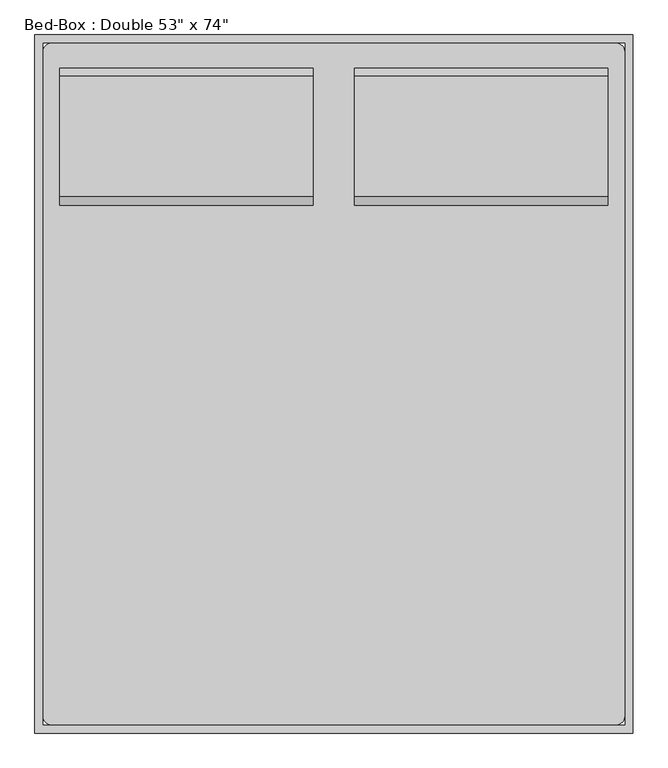
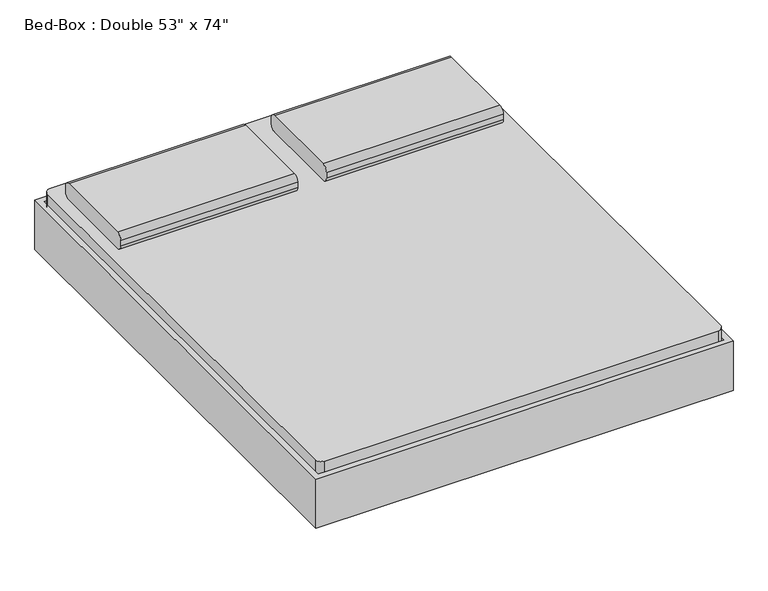
"""IFC4 building model written with IfcOpenShell, lengths in millimetres: furniture geometry."""

from ifc_helpers import new_model, si_unit, point, frame, frame_2d, origin, place, context, project, spatial, polyline, circle_curve, trimmed, segment, composite_curve, outline, extrude, source, transform, mapped, element, save
from ifc_brep_helpers import plane_surface, cylinder_surface, revolved_surface, advanced_brep


def furniture_2b620373(model_context):
    return source(origin(), model_context, "Body", "SolidModel", [
        extrude(outline(composite_curve([segment(polyline([(705.3704918, 406.4), (337.0704918, 406.4)]), True, "CONTINUOUS"), segment(trimmed(circle_curve(frame_2d((337.0704918, 431.8)), 25.4), [point((337.0704918, 406.4))], [point((311.6704918, 431.8))], False, "CARTESIAN"), True, "CONTINUOUS"), segment(polyline([(311.6704918, 431.8), (311.6704918, 457.2)]), True, "CONTINUOUS"), segment(trimmed(circle_curve(frame_2d((337.0704918, 457.2)), 25.4), [point((311.6704918, 457.2))], [point((337.0704918, 482.6))], False, "CARTESIAN"), True, "CONTINUOUS"), segment(polyline([(337.0704918, 482.6), (705.3704918, 482.6)]), True, "CONTINUOUS"), segment(trimmed(circle_curve(frame_2d((705.3704918, 457.2)), 25.4), [point((705.3704918, 482.6))], [point((730.7704918, 457.2))], False, "CARTESIAN"), True, "CONTINUOUS"), segment(polyline([(730.7704918, 457.2), (730.7704918, 431.8)]), True, "CONTINUOUS"), segment(trimmed(circle_curve(frame_2d((705.3704918, 431.8)), 25.4), [point((730.7704918, 431.8))], [point((705.3704918, 406.4))], False, "CARTESIAN"), True, "CONTINUOUS")], self_intersect=False)), frame((402.652459, 0.0, 0.0), z_axis=(1.0, 0.0, 0.0), x_axis=(0.0, 1.0, 0.0)), (0.0, 0.0, 1.0), 774.7),
        extrude(outline(composite_curve([segment(polyline([(705.3704918, 406.4), (337.0704918, 406.4)]), True, "CONTINUOUS"), segment(trimmed(circle_curve(frame_2d((337.0704918, 431.8)), 25.4), [point((337.0704918, 406.4))], [point((311.6704918, 431.8))], False, "CARTESIAN"), True, "CONTINUOUS"), segment(polyline([(311.6704918, 431.8), (311.6704918, 457.2)]), True, "CONTINUOUS"), segment(trimmed(circle_curve(frame_2d((337.0704918, 457.2)), 25.4), [point((311.6704918, 457.2))], [point((337.0704918, 482.6))], False, "CARTESIAN"), True, "CONTINUOUS"), segment(polyline([(337.0704918, 482.6), (705.3704918, 482.6)]), True, "CONTINUOUS"), segment(trimmed(circle_curve(frame_2d((705.3704918, 457.2)), 25.4), [point((705.3704918, 482.6))], [point((730.7704918, 457.2))], False, "CARTESIAN"), True, "CONTINUOUS"), segment(polyline([(730.7704918, 457.2), (730.7704918, 431.8)]), True, "CONTINUOUS"), segment(trimmed(circle_curve(frame_2d((705.3704918, 431.8)), 25.4), [point((730.7704918, 431.8))], [point((705.3704918, 406.4))], False, "CARTESIAN"), True, "CONTINUOUS")], self_intersect=False)), frame((-499.047541, 0.0, 0.0), z_axis=(1.0, 0.0, 0.0), x_axis=(0.0, 1.0, 0.0)), (0.0, 0.0, 1.0), 774.7),
        advanced_brep(
        [(-549.5231784, 578.3704918, 177.8), (-549.5231784, 502.1704918, 177.8), (-549.5231784, 502.1704918, 196.85), (-549.5231784, 578.3704918, 196.85), (-498.7231784, 578.3704918, 177.8), (-498.7231784, 502.1704918, 177.8), (-486.5869899, 502.1704918, 196.85), (-486.5869899, 578.3704918, 196.85), (-422.6523099, 578.3704918, 14.6654962), (-422.6523099, 502.1704918, 14.6654962), (-405.3871466, 502.1704918, 22.716374), (-405.3871466, 578.3704918, 22.716374), (-399.6320921, 502.1704918, 0.0), (-399.6320921, 578.3704918, 0.0), (-399.6320921, 502.1704918, 19.05), (-399.6320921, 578.3704918, 19.05), (-321.0195862, 578.3704918, 0.0), (-321.0195862, 502.1704918, 0.0), (-321.0195862, 502.1704918, 19.05), (-321.0195862, 578.3704918, 19.05), (-308.3195862, 502.1704918, 3.4029547), (-308.3195862, 578.3704918, 3.4029547), (-317.8445862, 502.1704918, 19.9007387), (-317.8445862, 578.3704918, 19.9007387), (-248.222541, 578.3704918, 38.1), (-248.222541, 502.1704918, 38.1), (-253.3269731, 502.1704918, 57.15), (-253.3269731, 578.3704918, 57.15), (926.8518216, 578.3704918, 38.1), (926.8518216, 502.1704918, 38.1), (931.9562537, 502.1704918, 57.15), (931.9562537, 578.3704918, 57.15), (986.9488669, 578.3704918, 3.4029547), (986.9488669, 502.1704918, 3.4029547), (996.4738669, 502.1704918, 19.9007387), (996.4738669, 578.3704918, 19.9007387), (999.6488669, 502.1704918, 0.0), (999.6488669, 578.3704918, 0.0), (999.6488669, 502.1704918, 19.05), (999.6488669, 578.3704918, 19.05), (1078.2613728, 578.3704918, 0.0), (1078.2613728, 502.1704918, 0.0), (1078.2613728, 502.1704918, 19.05), (1078.2613728, 578.3704918, 19.05), (1101.2815906, 502.1704918, 14.6654962), (1101.2815906, 578.3704918, 14.6654962), (1084.0164272, 502.1704918, 22.716374), (1084.0164272, 578.3704918, 22.716374), (1177.352459, 578.3704918, 177.8), (1177.352459, 502.1704918, 177.8), (1165.2162705, 502.1704918, 196.85), (1165.2162705, 578.3704918, 196.85), (1228.152459, 578.3704918, 177.8), (1228.152459, 578.3704918, 196.85), (1228.152459, 502.1704918, 196.85), (1228.152459, 502.1704918, 177.8)],
        [
            (0, 1),
            (1, 2),
            (2, 3),
            (3, 0),
            (0, 4),
            (4, 5),
            (5, 1),
            (5, 6),
            (6, 2),
            (6, 7),
            (7, 3),
            (7, 4),
            (4, 8),
            (8, 9),
            (9, 5),
            (9, 10),
            (10, 6),
            (10, 11),
            (11, 7),
            (11, 8),
            (12, 9, circle_curve(frame((-399.6320921, 502.1704918, 25.4), z_axis=(0.0, 1.0, 0.0), x_axis=(-0.9063077870366486, 0.0, -0.42261826174070233)), 25.4)),
            (8, 13, circle_curve(frame((-399.6320921, 578.3704918, 25.4), z_axis=(0.0, -1.0, 0.0), x_axis=(-0.9063077870366486, 0.0, -0.42261826174070233)), 25.4)),
            (13, 12),
            (14, 10, circle_curve(frame((-399.6320921, 502.1704918, 25.4), z_axis=(0.0, 1.0, 0.0), x_axis=(-0.9063077870366486, 0.0, -0.42261826174070233)), 6.35)),
            (12, 14),
            (15, 11, circle_curve(frame((-399.6320921, 578.3704918, 25.4), z_axis=(0.0, 1.0, 0.0), x_axis=(-0.9063077870366486, 0.0, -0.42261826174070233)), 6.35)),
            (14, 15),
            (15, 13),
            (13, 16),
            (16, 17),
            (17, 12),
            (17, 18),
            (18, 14),
            (18, 19),
            (19, 15),
            (19, 16),
            (20, 17, circle_curve(frame((-321.0195862, 502.1704918, 25.4), z_axis=(0.0, 1.0, 0.0), x_axis=(0.0, 0.0, -1.0)), 25.4)),
            (16, 21, circle_curve(frame((-321.0195862, 578.3704918, 25.4), z_axis=(0.0, -1.0, 0.0), x_axis=(0.0, 0.0, -1.0)), 25.4)),
            (21, 20),
            (22, 18, circle_curve(frame((-321.0195862, 502.1704918, 25.4), z_axis=(0.0, 1.0, 0.0), x_axis=(0.0, 0.0, -1.0)), 6.35)),
            (20, 22),
            (23, 19, circle_curve(frame((-321.0195862, 578.3704918, 25.4), z_axis=(0.0, 1.0, 0.0), x_axis=(0.0, 0.0, -1.0)), 6.35)),
            (22, 23),
            (23, 21),
            (21, 24),
            (24, 25),
            (25, 20),
            (25, 26),
            (26, 22),
            (26, 27),
            (27, 23),
            (27, 24),
            (24, 28),
            (28, 29),
            (29, 25),
            (29, 30),
            (30, 26),
            (30, 31),
            (31, 27),
            (31, 28),
            (28, 32),
            (32, 33),
            (33, 29),
            (33, 34),
            (34, 30),
            (34, 35),
            (35, 31),
            (35, 32),
            (36, 33, circle_curve(frame((999.6488669, 502.1704918, 25.4), z_axis=(0.0, 1.0, 0.0), x_axis=(-0.5000000000000463, 0.0, -0.8660254037844118)), 25.4)),
            (32, 37, circle_curve(frame((999.6488669, 578.3704918, 25.4), z_axis=(0.0, -1.0, 0.0), x_axis=(-0.5000000000000463, 0.0, -0.8660254037844118)), 25.4)),
            (37, 36),
            (38, 34, circle_curve(frame((999.6488669, 502.1704918, 25.4), z_axis=(0.0, 1.0, 0.0), x_axis=(-0.5000000000000463, 0.0, -0.8660254037844118)), 6.35)),
            (36, 38),
            (39, 35, circle_curve(frame((999.6488669, 578.3704918, 25.4), z_axis=(0.0, 1.0, 0.0), x_axis=(-0.5000000000000463, 0.0, -0.8660254037844118)), 6.35)),
            (38, 39),
            (39, 37),
            (37, 40),
            (40, 41),
            (41, 36),
            (41, 42),
            (42, 38),
            (42, 43),
            (43, 39),
            (43, 40),
            (44, 41, circle_curve(frame((1078.2613728, 502.1704918, 25.4), z_axis=(0.0, 1.0, 0.0), x_axis=(0.0, 0.0, -1.0)), 25.4)),
            (40, 45, circle_curve(frame((1078.2613728, 578.3704918, 25.4), z_axis=(0.0, -1.0, 0.0), x_axis=(0.0, 0.0, -1.0)), 25.4)),
            (45, 44),
            (46, 42, circle_curve(frame((1078.2613728, 502.1704918, 25.4), z_axis=(0.0, 1.0, 0.0), x_axis=(0.0, 0.0, -1.0)), 6.35)),
            (44, 46),
            (47, 43, circle_curve(frame((1078.2613728, 578.3704918, 25.4), z_axis=(0.0, 1.0, 0.0), x_axis=(0.0, 0.0, -1.0)), 6.35)),
            (46, 47),
            (47, 45),
            (45, 48),
            (48, 49),
            (49, 44),
            (49, 50),
            (50, 46),
            (50, 51),
            (51, 47),
            (51, 48),
            (52, 53),
            (53, 54),
            (54, 55),
            (55, 52),
            (48, 52),
            (55, 49),
            (54, 50),
            (53, 51),
        ],
        [
            plane_surface(frame((-549.5231784, 832.3704918, -152.9490627), z_axis=(-1.0, 0.0, 0.0), x_axis=(0.0, 1.0, 0.0))),
            plane_surface(frame((-549.5231784, 578.3704918, 177.8), z_axis=(0.0, 0.0, -1.0), x_axis=(1.0, 0.0, 0.0))),
            plane_surface(frame((-549.5231784, 502.1704918, 177.8), z_axis=(0.0, -1.0, 0.0), x_axis=(1.0, 0.0, 0.0))),
            plane_surface(frame((-549.5231784, 502.1704918, 196.85), z_axis=(0.0, 0.0, 1.0), x_axis=(1.0, 0.0, 0.0))),
            plane_surface(frame((-549.5231784, 578.3704918, 196.85), z_axis=(0.0, 1.0, 0.0), x_axis=(1.0, 0.0, 0.0))),
            plane_surface(frame((-498.7231784, 578.3704918, 177.8), z_axis=(-0.9063077870366487, 0.0, -0.4226182617407023), x_axis=(0.4226182617407023, 0.0, -0.9063077870366487))),
            plane_surface(frame((-498.7231784, 502.1704918, 177.8), z_axis=(0.0, -1.0000000000000002, 0.0), x_axis=(0.4226182617407023, 0.0, -0.9063077870366487))),
            plane_surface(frame((-486.5869899, 502.1704918, 196.85), z_axis=(0.9063077870366488, 0.0, 0.42261826174070205), x_axis=(0.42261826174070205, 0.0, -0.9063077870366488))),
            plane_surface(frame((-486.5869899, 578.3704918, 196.85), z_axis=(0.0, 1.0000000000000002, 0.0), x_axis=(0.4226182617407021, 0.0, -0.9063077870366487))),
            cylinder_surface(frame((-399.6320921, 832.3704918, 25.4), z_axis=(0.0, -1.0, 0.0), x_axis=(-0.9063077870366486, 0.0, -0.42261826174070233)), 25.4),
            plane_surface(frame((-399.6320921, 502.1704918, 25.4), z_axis=(0.0, -1.0, 0.0), x_axis=(-0.9063077870366486, 0.0, -0.42261826174070233))),
            revolved_surface(polyline([(-405.38714654768273, 502.1704918, 22.71637403794654), (-405.38714654768273, 578.3704918, 22.71637403794654)]), (-399.6320921, 832.3704918, 25.4), (0.0, -1.0, 0.0)),
            plane_surface(frame((-399.6320921, 578.3704918, 25.4), z_axis=(0.0, 1.0, 0.0), x_axis=(-0.9063077870366486, 0.0, -0.42261826174070233))),
            plane_surface(frame((-399.6320921, 578.3704918, 0.0), z_axis=(0.0, 0.0, -1.0), x_axis=(1.0, 0.0, 0.0))),
            plane_surface(frame((-399.6320921, 502.1704918, 0.0), z_axis=(0.0, -1.0, 0.0), x_axis=(1.0, 0.0, 0.0))),
            plane_surface(frame((-399.6320921, 502.1704918, 19.05), z_axis=(0.0, 0.0, 1.0), x_axis=(1.0, 0.0, 0.0))),
            plane_surface(frame((-399.6320921, 578.3704918, 19.05), z_axis=(0.0, 1.0, 0.0), x_axis=(1.0, 0.0, 0.0))),
            cylinder_surface(frame((-321.0195862, 832.3704918, 25.4), z_axis=(0.0, -1.0, 0.0), x_axis=(0.0, 0.0, -1.0)), 25.4),
            plane_surface(frame((-321.0195862, 502.1704918, 25.4), z_axis=(0.0, -1.0, 0.0), x_axis=(0.0, 0.0, -1.0))),
            revolved_surface(polyline([(-321.0195862, 502.1704918, 19.049999999999997), (-321.0195862, 578.3704918, 19.049999999999997)]), (-321.0195862, 832.3704918, 25.4), (0.0, -1.0, 0.0)),
            plane_surface(frame((-321.0195862, 578.3704918, 25.4), z_axis=(0.0, 1.0, 0.0), x_axis=(0.0, 0.0, -1.0))),
            plane_surface(frame((-308.3195862, 578.3704918, 3.4029547), z_axis=(0.49999999999987804, 0.0, -0.8660254037845091), x_axis=(0.8660254037845091, 0.0, 0.49999999999987804))),
            plane_surface(frame((-308.3195862, 502.1704918, 3.4029547), z_axis=(0.0, -1.0000000000000002, 0.0), x_axis=(0.8660254037845095, 0.0, 0.4999999999998774))),
            plane_surface(frame((-317.8445862, 502.1704918, 19.9007387), z_axis=(-0.49999999999987743, 0.0, 0.8660254037845095), x_axis=(0.8660254037845095, 0.0, 0.49999999999987743))),
            plane_surface(frame((-317.8445862, 578.3704918, 19.9007387), z_axis=(0.0, 1.0, 0.0), x_axis=(0.8660254037845087, 0.0, 0.49999999999987876))),
            plane_surface(frame((-248.222541, 578.3704918, 38.1), z_axis=(0.0, 0.0, -1.0), x_axis=(1.0, 0.0, 0.0))),
            plane_surface(frame((-248.222541, 502.1704918, 38.1), z_axis=(0.0, -1.0, 0.0), x_axis=(1.0, 0.0, 0.0))),
            plane_surface(frame((-253.3269731, 502.1704918, 57.15), z_axis=(0.0, 0.0, 1.0), x_axis=(1.0, 0.0, 0.0))),
            plane_surface(frame((-253.3269731, 578.3704918, 57.15), z_axis=(0.0, 1.0, 0.0), x_axis=(1.0, 0.0, 0.0))),
            plane_surface(frame((926.8518216, 578.3704918, 38.1), z_axis=(-0.5000000000000462, 0.0, -0.866025403784412), x_axis=(0.866025403784412, 0.0, -0.5000000000000462))),
            plane_surface(frame((926.8518216, 502.1704918, 38.1), z_axis=(0.0, -1.0, 0.0), x_axis=(0.8660254037844121, 0.0, -0.5000000000000461))),
            plane_surface(frame((931.9562537, 502.1704918, 57.15), z_axis=(0.5000000000000455, 0.0, 0.8660254037844124), x_axis=(0.8660254037844124, 0.0, -0.5000000000000455))),
            plane_surface(frame((931.9562537, 578.3704918, 57.15), z_axis=(0.0, 1.0, 0.0), x_axis=(0.866025403784413, 0.0, -0.5000000000000446))),
            cylinder_surface(frame((999.6488669, 832.3704918, 25.4), z_axis=(0.0, -1.0, 0.0), x_axis=(-0.5000000000000463, 0.0, -0.8660254037844118)), 25.4),
            plane_surface(frame((999.6488669, 502.1704918, 25.4), z_axis=(0.0, -1.0000000000000002, 0.0), x_axis=(-0.5000000000000464, 0.0, -0.866025403784412))),
            revolved_surface(polyline([(996.4738668999997, 502.1704918, 19.90073868596898), (996.4738668999997, 578.3704918, 19.90073868596898)]), (999.6488669, 832.3704918, 25.4), (0.0, -1.0, 0.0)),
            plane_surface(frame((999.6488669, 578.3704918, 25.4), z_axis=(0.0, 1.0000000000000002, 0.0), x_axis=(-0.5000000000000464, 0.0, -0.866025403784412))),
            plane_surface(frame((999.6488669, 578.3704918, 0.0), z_axis=(0.0, 0.0, -1.0), x_axis=(1.0, 0.0, 0.0))),
            plane_surface(frame((999.6488669, 502.1704918, 0.0), z_axis=(0.0, -1.0, 0.0), x_axis=(1.0, 0.0, 0.0))),
            plane_surface(frame((999.6488669, 502.1704918, 19.05), z_axis=(0.0, 0.0, 1.0), x_axis=(1.0, 0.0, 0.0))),
            plane_surface(frame((999.6488669, 578.3704918, 19.05), z_axis=(0.0, 1.0, 0.0), x_axis=(1.0, 0.0, 0.0))),
            cylinder_surface(frame((1078.2613728, 832.3704918, 25.4), z_axis=(0.0, -1.0, 0.0), x_axis=(0.0, 0.0, -1.0)), 25.4),
            plane_surface(frame((1078.2613728, 502.1704918, 25.4), z_axis=(0.0, -1.0, 0.0), x_axis=(0.0, 0.0, -1.0))),
            revolved_surface(polyline([(1078.2613728, 502.1704918, 19.049999999999997), (1078.2613728, 578.3704918, 19.049999999999997)]), (1078.2613728, 832.3704918, 25.4), (0.0, -1.0, 0.0)),
            plane_surface(frame((1078.2613728, 578.3704918, 25.4), z_axis=(0.0, 1.0, 0.0), x_axis=(0.0, 0.0, -1.0))),
            plane_surface(frame((1101.2815906, 578.3704918, 14.6654962), z_axis=(0.90630778703668, 0.0, -0.422618261740635), x_axis=(0.422618261740635, 0.0, 0.90630778703668))),
            plane_surface(frame((1101.2815906, 502.1704918, 14.6654962), z_axis=(0.0, -1.0000000000000002, 0.0), x_axis=(0.4226182617406349, 0.0, 0.9063077870366801))),
            plane_surface(frame((1084.0164272, 502.1704918, 22.716374), z_axis=(-0.9063077870366799, 0.0, 0.4226182617406352), x_axis=(0.4226182617406352, 0.0, 0.9063077870366799))),
            plane_surface(frame((1084.0164272, 578.3704918, 22.716374), z_axis=(0.0, 1.0, 0.0), x_axis=(0.42261826174063544, 0.0, 0.9063077870366798))),
            plane_surface(frame((1228.152459, 832.3704918, -152.9490627), z_axis=(1.0, 0.0, 0.0), x_axis=(0.0, 1.0, 0.0))),
            plane_surface(frame((1177.352459, 578.3704918, 177.8), z_axis=(0.0, 0.0, -1.0), x_axis=(1.0, 0.0, 0.0))),
            plane_surface(frame((1177.352459, 502.1704918, 177.8), z_axis=(0.0, -1.0, 0.0), x_axis=(1.0, 0.0, 0.0))),
            plane_surface(frame((1165.2162705, 502.1704918, 196.85), z_axis=(0.0, 0.0, 1.0), x_axis=(1.0, 0.0, 0.0))),
            plane_surface(frame((1165.2162705, 578.3704918, 196.85), z_axis=(0.0, 1.0, 0.0), x_axis=(1.0, 0.0, 0.0))),
        ],
        [
            (0, [[1, 2, 3, 4]]),
            (1, [[-1, 5, 6, 7]]),
            (2, [[-2, -7, 8, 9]]),
            (3, [[-3, -9, 10, 11]]),
            (4, [[-4, -11, 12, -5]]),
            (5, [[-6, 13, 14, 15]]),
            (6, [[-8, -15, 16, 17]]),
            (7, [[-10, -17, 18, 19]]),
            (8, [[-12, -19, 20, -13]]),
            (9, [[21, -14, 22, 23]]),
            (10, [[24, -16, -21, 25]]),
            (11, [[26, -18, -24, 27]]),
            (12, [[-22, -20, -26, 28]]),
            (13, [[-23, 29, 30, 31]]),
            (14, [[-25, -31, 32, 33]]),
            (15, [[-27, -33, 34, 35]]),
            (16, [[-28, -35, 36, -29]]),
            (17, [[37, -30, 38, 39]]),
            (18, [[40, -32, -37, 41]]),
            (19, [[42, -34, -40, 43]]),
            (20, [[-38, -36, -42, 44]]),
            (21, [[-39, 45, 46, 47]]),
            (22, [[-41, -47, 48, 49]]),
            (23, [[-43, -49, 50, 51]]),
            (24, [[-44, -51, 52, -45]]),
            (25, [[-46, 53, 54, 55]]),
            (26, [[-48, -55, 56, 57]]),
            (27, [[-50, -57, 58, 59]]),
            (28, [[-52, -59, 60, -53]]),
            (29, [[-54, 61, 62, 63]]),
            (30, [[-56, -63, 64, 65]]),
            (31, [[-58, -65, 66, 67]]),
            (32, [[-60, -67, 68, -61]]),
            (33, [[69, -62, 70, 71]]),
            (34, [[72, -64, -69, 73]]),
            (35, [[74, -66, -72, 75]]),
            (36, [[-70, -68, -74, 76]]),
            (37, [[-71, 77, 78, 79]]),
            (38, [[-73, -79, 80, 81]]),
            (39, [[-75, -81, 82, 83]]),
            (40, [[-76, -83, 84, -77]]),
            (41, [[85, -78, 86, 87]]),
            (42, [[88, -80, -85, 89]]),
            (43, [[90, -82, -88, 91]]),
            (44, [[-86, -84, -90, 92]]),
            (45, [[-87, 93, 94, 95]]),
            (46, [[-89, -95, 96, 97]]),
            (47, [[-91, -97, 98, 99]]),
            (48, [[-92, -99, 100, -93]]),
            (49, [[101, 102, 103, 104]]),
            (50, [[-94, 105, -104, 106]]),
            (51, [[-96, -106, -103, 107]]),
            (52, [[-98, -107, -102, 108]]),
            (53, [[-100, -108, -101, -105]]),
        ],
    ),
        extrude(outline(composite_curve([segment(polyline([(-524.447541, 806.9704918), (1202.752459, 806.9704918)]), True, "CONTINUOUS"), segment(trimmed(circle_curve(frame_2d((1202.752459, 781.5704918)), 25.4), [point((1202.752459, 806.9704918))], [point((1228.152459, 781.5704918))], False, "CARTESIAN"), True, "CONTINUOUS"), segment(polyline([(1228.152459, 781.5704918), (1228.152459, -1250.4295082)]), True, "CONTINUOUS"), segment(trimmed(circle_curve(frame_2d((1202.752459, -1250.4295082)), 25.4), [point((1228.152459, -1250.4295082))], [point((1202.752459, -1275.8295082))], False, "CARTESIAN"), True, "CONTINUOUS"), segment(polyline([(1202.752459, -1275.8295082), (-524.447541, -1275.8295082)]), True, "CONTINUOUS"), segment(trimmed(circle_curve(frame_2d((-524.447541, -1250.4295082)), 25.4), [point((-524.447541, -1275.8295082))], [point((-549.847541, -1250.4295082))], False, "CARTESIAN"), True, "CONTINUOUS"), segment(polyline([(-549.847541, -1250.4295082), (-549.847541, 781.5704918)]), True, "CONTINUOUS"), segment(trimmed(circle_curve(frame_2d((-524.447541, 781.5704918)), 25.4), [point((-549.847541, 781.5704918))], [point((-524.447541, 806.9704918))], False, "CARTESIAN"), True, "CONTINUOUS")], self_intersect=False)), frame((0.0, 0.0, 203.2), z_axis=(0.0, 0.0, 1.0), x_axis=(1.0, 0.0, 0.0)), (0.0, 0.0, 1.0), 203.2),
        advanced_brep(
        [(-549.847541, -996.4295082, 196.85), (-549.847541, -996.4295082, 177.8), (-549.847541, -1072.6295082, 177.8), (-549.847541, -1072.6295082, 196.85), (-486.9113525, -996.4295082, 196.85), (-499.047541, -996.4295082, 177.8), (-499.047541, -1072.6295082, 177.8), (-486.9113525, -1072.6295082, 196.85), (-405.7115092, -996.4295082, 22.716374), (-422.9766725, -996.4295082, 14.6654962), (-422.9766725, -1072.6295082, 14.6654962), (-405.7115092, -1072.6295082, 22.716374), (-399.9564547, -996.4295082, 0.0), (-399.9564547, -996.4295082, 19.05), (-399.9564547, -1072.6295082, 0.0), (-399.9564547, -1072.6295082, 19.05), (-321.3439489, -996.4295082, 19.05), (-321.3439489, -996.4295082, 0.0), (-321.3439489, -1072.6295082, 0.0), (-321.3439489, -1072.6295082, 19.05), (-308.6439489, -996.4295082, 3.4029547), (-318.1689489, -996.4295082, 19.9007387), (-308.6439489, -1072.6295082, 3.4029547), (-318.1689489, -1072.6295082, 19.9007387), (-253.6513357, -996.4295082, 57.15), (-248.5469036, -996.4295082, 38.1), (-248.5469036, -1072.6295082, 38.1), (-253.6513357, -1072.6295082, 57.15), (931.9562537, -996.4295082, 57.15), (926.8518216, -996.4295082, 38.1), (926.8518216, -1072.6295082, 38.1), (931.9562537, -1072.6295082, 57.15), (996.4738669, -996.4295082, 19.9007387), (986.9488669, -996.4295082, 3.4029547), (986.9488669, -1072.6295082, 3.4029547), (996.4738669, -1072.6295082, 19.9007387), (999.6488669, -996.4295082, 0.0), (999.6488669, -996.4295082, 19.05), (999.6488669, -1072.6295082, 0.0), (999.6488669, -1072.6295082, 19.05), (1078.2613728, -996.4295082, 19.05), (1078.2613728, -996.4295082, 0.0), (1078.2613728, -1072.6295082, 0.0), (1078.2613728, -1072.6295082, 19.05), (1101.2815906, -996.4295082, 14.6654962), (1084.0164272, -996.4295082, 22.716374), (1101.2815906, -1072.6295082, 14.6654962), (1084.0164272, -1072.6295082, 22.716374), (1165.2162705, -996.4295082, 196.85), (1177.352459, -996.4295082, 177.8), (1177.352459, -1072.6295082, 177.8), (1165.2162705, -1072.6295082, 196.85), (1228.152459, -996.4295082, 196.85), (1228.152459, -1072.6295082, 196.85), (1228.152459, -1072.6295082, 177.8), (1228.152459, -996.4295082, 177.8)],
        [
            (0, 1),
            (1, 2),
            (2, 3),
            (3, 0),
            (0, 4),
            (4, 5),
            (5, 1),
            (5, 6),
            (6, 2),
            (6, 7),
            (7, 3),
            (7, 4),
            (4, 8),
            (8, 9),
            (9, 5),
            (9, 10),
            (10, 6),
            (10, 11),
            (11, 7),
            (11, 8),
            (12, 9, circle_curve(frame((-399.9564547, -996.4295082, 25.4), z_axis=(0.0, 1.0, 0.0), x_axis=(-0.906307787036663, 0.0, -0.4226182617406713)), 25.4)),
            (8, 13, circle_curve(frame((-399.9564547, -996.4295082, 25.4), z_axis=(0.0, -1.0, 0.0), x_axis=(-0.906307787036663, 0.0, -0.4226182617406713)), 6.35)),
            (13, 12),
            (14, 10, circle_curve(frame((-399.9564547, -1072.6295082, 25.4), z_axis=(0.0, 1.0, 0.0), x_axis=(-0.906307787036663, 0.0, -0.4226182617406713)), 25.4)),
            (12, 14),
            (15, 11, circle_curve(frame((-399.9564547, -1072.6295082, 25.4), z_axis=(0.0, 1.0, 0.0), x_axis=(-0.906307787036663, 0.0, -0.4226182617406713)), 6.35)),
            (14, 15),
            (15, 13),
            (13, 16),
            (16, 17),
            (17, 12),
            (17, 18),
            (18, 14),
            (18, 19),
            (19, 15),
            (19, 16),
            (20, 17, circle_curve(frame((-321.3439489, -996.4295082, 25.4), z_axis=(0.0, 1.0, 0.0), x_axis=(0.0, 0.0, -1.0)), 25.4)),
            (16, 21, circle_curve(frame((-321.3439489, -996.4295082, 25.4), z_axis=(0.0, -1.0, 0.0), x_axis=(0.0, 0.0, -1.0)), 6.35)),
            (21, 20),
            (22, 18, circle_curve(frame((-321.3439489, -1072.6295082, 25.4), z_axis=(0.0, 1.0, 0.0), x_axis=(0.0, 0.0, -1.0)), 25.4)),
            (20, 22),
            (23, 19, circle_curve(frame((-321.3439489, -1072.6295082, 25.4), z_axis=(0.0, 1.0, 0.0), x_axis=(0.0, 0.0, -1.0)), 6.35)),
            (22, 23),
            (23, 21),
            (21, 24),
            (24, 25),
            (25, 20),
            (25, 26),
            (26, 22),
            (26, 27),
            (27, 23),
            (27, 24),
            (24, 28),
            (28, 29),
            (29, 25),
            (29, 30),
            (30, 26),
            (30, 31),
            (31, 27),
            (31, 28),
            (28, 32),
            (32, 33),
            (33, 29),
            (33, 34),
            (34, 30),
            (34, 35),
            (35, 31),
            (35, 32),
            (36, 33, circle_curve(frame((999.6488669, -996.4295082, 25.4), z_axis=(0.0, 1.0, 0.0), x_axis=(-0.5000000000000479, 0.0, -0.866025403784411)), 25.4)),
            (32, 37, circle_curve(frame((999.6488669, -996.4295082, 25.4), z_axis=(0.0, -1.0, 0.0), x_axis=(-0.5000000000000479, 0.0, -0.866025403784411)), 6.35)),
            (37, 36),
            (38, 34, circle_curve(frame((999.6488669, -1072.6295082, 25.4), z_axis=(0.0, 1.0, 0.0), x_axis=(-0.5000000000000479, 0.0, -0.866025403784411)), 25.4)),
            (36, 38),
            (39, 35, circle_curve(frame((999.6488669, -1072.6295082, 25.4), z_axis=(0.0, 1.0, 0.0), x_axis=(-0.5000000000000479, 0.0, -0.866025403784411)), 6.35)),
            (38, 39),
            (39, 37),
            (37, 40),
            (40, 41),
            (41, 36),
            (41, 42),
            (42, 38),
            (42, 43),
            (43, 39),
            (43, 40),
            (44, 41, circle_curve(frame((1078.2613728, -996.4295082, 25.4), z_axis=(0.0, 1.0, 0.0), x_axis=(0.0, 0.0, -1.0)), 25.4)),
            (40, 45, circle_curve(frame((1078.2613728, -996.4295082, 25.4), z_axis=(0.0, -1.0, 0.0), x_axis=(0.0, 0.0, -1.0)), 6.35)),
            (45, 44),
            (46, 42, circle_curve(frame((1078.2613728, -1072.6295082, 25.4), z_axis=(0.0, 1.0, 0.0), x_axis=(0.0, 0.0, -1.0)), 25.4)),
            (44, 46),
            (47, 43, circle_curve(frame((1078.2613728, -1072.6295082, 25.4), z_axis=(0.0, 1.0, 0.0), x_axis=(0.0, 0.0, -1.0)), 6.35)),
            (46, 47),
            (47, 45),
            (45, 48),
            (48, 49),
            (49, 44),
            (49, 50),
            (50, 46),
            (50, 51),
            (51, 47),
            (51, 48),
            (52, 53),
            (53, 54),
            (54, 55),
            (55, 52),
            (48, 52),
            (55, 49),
            (54, 50),
            (53, 51),
        ],
        [
            plane_surface(frame((-549.847541, -1301.2295082, -127.5947323), z_axis=(-1.0, 0.0, 0.0), x_axis=(0.0, 1.0, 0.0))),
            plane_surface(frame((-549.847541, -996.4295082, 196.85), z_axis=(0.0, 1.0, 0.0), x_axis=(1.0, 0.0, 0.0))),
            plane_surface(frame((-549.847541, -996.4295082, 177.8), z_axis=(0.0, 0.0, -1.0), x_axis=(1.0, 0.0, 0.0))),
            plane_surface(frame((-549.847541, -1072.6295082, 177.8), z_axis=(0.0, -1.0, 0.0), x_axis=(1.0, 0.0, 0.0))),
            plane_surface(frame((-549.847541, -1072.6295082, 196.85), z_axis=(0.0, 0.0, 1.0), x_axis=(1.0, 0.0, 0.0))),
            plane_surface(frame((-486.9113525, -996.4295082, 196.85), z_axis=(0.0, 1.0, 0.0), x_axis=(0.42261826174067074, 0.0, -0.9063077870366634))),
            plane_surface(frame((-499.047541, -996.4295082, 177.8), z_axis=(-0.9063077870366634, 0.0, -0.4226182617406708), x_axis=(0.4226182617406708, 0.0, -0.9063077870366634))),
            plane_surface(frame((-499.047541, -1072.6295082, 177.8), z_axis=(0.0, -1.0, 0.0), x_axis=(0.4226182617406708, 0.0, -0.9063077870366634))),
            plane_surface(frame((-486.9113525, -1072.6295082, 196.85), z_axis=(0.9063077870366634, 0.0, 0.42261826174067074), x_axis=(0.42261826174067074, 0.0, -0.9063077870366634))),
            plane_surface(frame((-399.9564547, -996.4295082, 25.4), z_axis=(0.0, 1.0, 0.0), x_axis=(-0.906307787036663, 0.0, -0.4226182617406713))),
            cylinder_surface(frame((-399.9564547, -1301.2295082, 25.4), z_axis=(0.0, -1.0, 0.0), x_axis=(-0.906307787036663, 0.0, -0.4226182617406713)), 25.4),
            plane_surface(frame((-399.9564547, -1072.6295082, 25.4), z_axis=(0.0, -1.0, 0.0), x_axis=(-0.906307787036663, 0.0, -0.4226182617406713))),
            revolved_surface(polyline([(-405.7115091476828, -1072.6295082, 22.716374037946736), (-405.7115091476828, -996.4295082, 22.716374037946736)]), (-399.9564547, -1301.2295082, 25.4), (0.0, -1.0, 0.0)),
            plane_surface(frame((-399.9564547, -996.4295082, 19.05), z_axis=(0.0, 1.0, 0.0), x_axis=(1.0, 0.0, 0.0))),
            plane_surface(frame((-399.9564547, -996.4295082, 0.0), z_axis=(0.0, 0.0, -1.0), x_axis=(1.0, 0.0, 0.0))),
            plane_surface(frame((-399.9564547, -1072.6295082, 0.0), z_axis=(0.0, -1.0, 0.0), x_axis=(1.0, 0.0, 0.0))),
            plane_surface(frame((-399.9564547, -1072.6295082, 19.05), z_axis=(0.0, 0.0, 1.0), x_axis=(1.0, 0.0, 0.0))),
            plane_surface(frame((-321.3439489, -996.4295082, 25.4), z_axis=(0.0, 1.0, 0.0), x_axis=(0.0, 0.0, -1.0))),
            cylinder_surface(frame((-321.3439489, -1301.2295082, 25.4), z_axis=(0.0, -1.0, 0.0), x_axis=(0.0, 0.0, -1.0)), 25.4),
            plane_surface(frame((-321.3439489, -1072.6295082, 25.4), z_axis=(0.0, -1.0, 0.0), x_axis=(0.0, 0.0, -1.0))),
            revolved_surface(polyline([(-321.3439489, -1072.6295082, 19.049999999999997), (-321.3439489, -996.4295082, 19.049999999999997)]), (-321.3439489, -1301.2295082, 25.4), (0.0, -1.0, 0.0)),
            plane_surface(frame((-318.1689489, -996.4295082, 19.9007387), z_axis=(0.0, 1.0, 0.0), x_axis=(0.8660254037844788, 0.0, 0.49999999999993056))),
            plane_surface(frame((-308.6439489, -996.4295082, 3.4029547), z_axis=(0.49999999999993083, 0.0, -0.8660254037844787), x_axis=(0.8660254037844787, 0.0, 0.49999999999993083))),
            plane_surface(frame((-308.6439489, -1072.6295082, 3.4029547), z_axis=(0.0, -1.0, 0.0), x_axis=(0.8660254037844791, 0.0, 0.49999999999992994))),
            plane_surface(frame((-318.1689489, -1072.6295082, 19.9007387), z_axis=(-0.4999999999999306, 0.0, 0.8660254037844788), x_axis=(0.8660254037844788, 0.0, 0.4999999999999306))),
            plane_surface(frame((-253.6513357, -996.4295082, 57.15), z_axis=(0.0, 1.0, 0.0), x_axis=(1.0, 0.0, 0.0))),
            plane_surface(frame((-248.5469036, -996.4295082, 38.1), z_axis=(0.0, 0.0, -1.0), x_axis=(1.0, 0.0, 0.0))),
            plane_surface(frame((-248.5469036, -1072.6295082, 38.1), z_axis=(0.0, -1.0, 0.0), x_axis=(1.0, 0.0, 0.0))),
            plane_surface(frame((-253.6513357, -1072.6295082, 57.15), z_axis=(0.0, 0.0, 1.0), x_axis=(1.0, 0.0, 0.0))),
            plane_surface(frame((931.9562537, -996.4295082, 57.15), z_axis=(0.0, 1.0, 0.0), x_axis=(0.8660254037844098, 0.0, -0.50000000000005))),
            plane_surface(frame((926.8518216, -996.4295082, 38.1), z_axis=(-0.5000000000000508, 0.0, -0.8660254037844093), x_axis=(0.8660254037844093, 0.0, -0.5000000000000508))),
            plane_surface(frame((926.8518216, -1072.6295082, 38.1), z_axis=(0.0, -1.0, 0.0), x_axis=(0.8660254037844096, 0.0, -0.5000000000000504))),
            plane_surface(frame((931.9562537, -1072.6295082, 57.15), z_axis=(0.5000000000000512, 0.0, 0.8660254037844092), x_axis=(0.8660254037844092, 0.0, -0.5000000000000512))),
            plane_surface(frame((999.6488669, -996.4295082, 25.4), z_axis=(0.0, 1.0000000000000002, 0.0), x_axis=(-0.500000000000048, 0.0, -0.8660254037844111))),
            cylinder_surface(frame((999.6488669, -1301.2295082, 25.4), z_axis=(0.0, -1.0, 0.0), x_axis=(-0.5000000000000479, 0.0, -0.866025403784411)), 25.4),
            plane_surface(frame((999.6488669, -1072.6295082, 25.4), z_axis=(0.0, -1.0000000000000002, 0.0), x_axis=(-0.500000000000048, 0.0, -0.8660254037844111))),
            revolved_surface(polyline([(996.4738668999997, -1072.6295082, 19.90073868596899), (996.4738668999997, -996.4295082, 19.90073868596899)]), (999.6488669, -1301.2295082, 25.4), (0.0, -1.0, 0.0)),
            plane_surface(frame((999.6488669, -996.4295082, 19.05), z_axis=(0.0, 1.0, 0.0), x_axis=(1.0, 0.0, 0.0))),
            plane_surface(frame((999.6488669, -996.4295082, 0.0), z_axis=(0.0, 0.0, -1.0), x_axis=(1.0, 0.0, 0.0))),
            plane_surface(frame((999.6488669, -1072.6295082, 0.0), z_axis=(0.0, -1.0, 0.0), x_axis=(1.0, 0.0, 0.0))),
            plane_surface(frame((999.6488669, -1072.6295082, 19.05), z_axis=(0.0, 0.0, 1.0), x_axis=(1.0, 0.0, 0.0))),
            plane_surface(frame((1078.2613728, -996.4295082, 25.4), z_axis=(0.0, 1.0, 0.0), x_axis=(0.0, 0.0, -1.0))),
            cylinder_surface(frame((1078.2613728, -1301.2295082, 25.4), z_axis=(0.0, -1.0, 0.0), x_axis=(0.0, 0.0, -1.0)), 25.4),
            plane_surface(frame((1078.2613728, -1072.6295082, 25.4), z_axis=(0.0, -1.0, 0.0), x_axis=(0.0, 0.0, -1.0))),
            revolved_surface(polyline([(1078.2613728, -1072.6295082, 19.049999999999997), (1078.2613728, -996.4295082, 19.049999999999997)]), (1078.2613728, -1301.2295082, 25.4), (0.0, -1.0, 0.0)),
            plane_surface(frame((1084.0164272, -996.4295082, 22.716374), z_axis=(0.0, 1.0, 0.0), x_axis=(0.4226182617405415, 0.0, 0.9063077870367237))),
            plane_surface(frame((1101.2815906, -996.4295082, 14.6654962), z_axis=(0.9063077870367237, 0.0, -0.4226182617405414), x_axis=(0.4226182617405414, 0.0, 0.9063077870367237))),
            plane_surface(frame((1101.2815906, -1072.6295082, 14.6654962), z_axis=(0.0, -1.0000000000000002, 0.0), x_axis=(0.42261826174054096, 0.0, 0.906307787036724))),
            plane_surface(frame((1084.0164272, -1072.6295082, 22.716374), z_axis=(-0.9063077870367237, 0.0, 0.4226182617405414), x_axis=(0.4226182617405414, 0.0, 0.9063077870367237))),
            plane_surface(frame((1228.152459, -1301.2295082, -127.5947323), z_axis=(1.0, 0.0, 0.0), x_axis=(0.0, 1.0, 0.0))),
            plane_surface(frame((1165.2162705, -996.4295082, 196.85), z_axis=(0.0, 1.0, 0.0), x_axis=(1.0, 0.0, 0.0))),
            plane_surface(frame((1177.352459, -996.4295082, 177.8), z_axis=(0.0, 0.0, -1.0), x_axis=(1.0, 0.0, 0.0))),
            plane_surface(frame((1177.352459, -1072.6295082, 177.8), z_axis=(0.0, -1.0, 0.0), x_axis=(1.0, 0.0, 0.0))),
            plane_surface(frame((1165.2162705, -1072.6295082, 196.85), z_axis=(0.0, 0.0, 1.0), x_axis=(1.0, 0.0, 0.0))),
        ],
        [
            (0, [[1, 2, 3, 4]]),
            (1, [[-1, 5, 6, 7]]),
            (2, [[-2, -7, 8, 9]]),
            (3, [[-3, -9, 10, 11]]),
            (4, [[-4, -11, 12, -5]]),
            (5, [[-6, 13, 14, 15]]),
            (6, [[-8, -15, 16, 17]]),
            (7, [[-10, -17, 18, 19]]),
            (8, [[-12, -19, 20, -13]]),
            (9, [[21, -14, 22, 23]]),
            (10, [[24, -16, -21, 25]]),
            (11, [[26, -18, -24, 27]]),
            (12, [[-22, -20, -26, 28]]),
            (13, [[-23, 29, 30, 31]]),
            (14, [[-25, -31, 32, 33]]),
            (15, [[-27, -33, 34, 35]]),
            (16, [[-28, -35, 36, -29]]),
            (17, [[37, -30, 38, 39]]),
            (18, [[40, -32, -37, 41]]),
            (19, [[42, -34, -40, 43]]),
            (20, [[-38, -36, -42, 44]]),
            (21, [[-39, 45, 46, 47]]),
            (22, [[-41, -47, 48, 49]]),
            (23, [[-43, -49, 50, 51]]),
            (24, [[-44, -51, 52, -45]]),
            (25, [[-46, 53, 54, 55]]),
            (26, [[-48, -55, 56, 57]]),
            (27, [[-50, -57, 58, 59]]),
            (28, [[-52, -59, 60, -53]]),
            (29, [[-54, 61, 62, 63]]),
            (30, [[-56, -63, 64, 65]]),
            (31, [[-58, -65, 66, 67]]),
            (32, [[-60, -67, 68, -61]]),
            (33, [[69, -62, 70, 71]]),
            (34, [[72, -64, -69, 73]]),
            (35, [[74, -66, -72, 75]]),
            (36, [[-70, -68, -74, 76]]),
            (37, [[-71, 77, 78, 79]]),
            (38, [[-73, -79, 80, 81]]),
            (39, [[-75, -81, 82, 83]]),
            (40, [[-76, -83, 84, -77]]),
            (41, [[85, -78, 86, 87]]),
            (42, [[88, -80, -85, 89]]),
            (43, [[90, -82, -88, 91]]),
            (44, [[-86, -84, -90, 92]]),
            (45, [[-87, 93, 94, 95]]),
            (46, [[-89, -95, 96, 97]]),
            (47, [[-91, -97, 98, 99]]),
            (48, [[-92, -99, 100, -93]]),
            (49, [[101, 102, 103, 104]]),
            (50, [[-94, 105, -104, 106]]),
            (51, [[-96, -106, -103, 107]]),
            (52, [[-98, -107, -102, 108]]),
            (53, [[-100, -108, -101, -105]]),
        ],
    ),
        extrude(outline(polyline([(1253.552459, 832.3704918), (1253.552459, -1301.2295082), (-575.247541, -1301.2295082), (-575.247541, 832.3704918), (1253.552459, 832.3704918)]), holes=[polyline([(1228.152459, 806.9704918), (-549.847541, 806.9704918), (-549.847541, -1275.8295082), (1228.152459, -1275.8295082), (1228.152459, 806.9704918)])]), frame((0.0, 0.0, 127.0), z_axis=(0.0, 0.0, 1.0), x_axis=(1.0, 0.0, 0.0)), (0.0, 0.0, 1.0), 228.6),
    ])


if __name__ == "__main__":
    model = new_model("IFC4")
    model_context = context("Model", 3, world=origin())
    ifc_project = project(units=[si_unit("LENGTHUNIT", "METRE", prefix="MILLI")], contexts=[model_context])
    site = spatial("IfcSite", under=ifc_project)
    building = spatial("IfcBuilding", under=site)
    placement = place(None, origin())
    furniture_shape = furniture_2b620373(model_context)
    element("IfcFurniture", 1, ObjectType="Bed-Box : Double 53\" x 74\"", at=placement, inside=building, context=model_context, shape_type="MappedRepresentation", body=[
        mapped(furniture_shape, transform((0.0, 0.0, 0.0), x_axis=(1.0, 0.0, 0.0), y_axis=(0.0, 1.0, 0.0), z_axis=(0.0, 0.0, 1.0))),
    ])
    save(model, "model.ifc")

# Revit data of these elements
# Type "Bed-Box : Double 53\" x 74\""
#   Assembly Code = "E2020200"
#   Length = 7' - 0"
#   Width = 6' - 0"
#   Frame Material = Birch
#   Mattress Material = Linen, White
#   Default Elevation = 0
# Element 1 (IfcFurniture, "Bed-Box : Double 53\" x 74\"")
#   Materials on its faces: "Birch", "Linen, White"
# Materials
#   "Birch": class "Wood", colour RGB 224 178 126, transparency 0, Description = "Betula Alleghaniensis", Cost = 0
#   "Linen, White": class "Textile", colour RGB 247 247 239, transparency 0, Description = "Linen, white", Cost = 0
